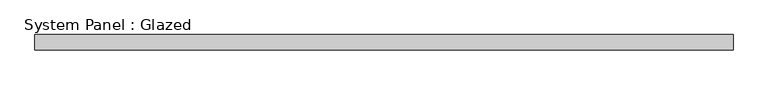
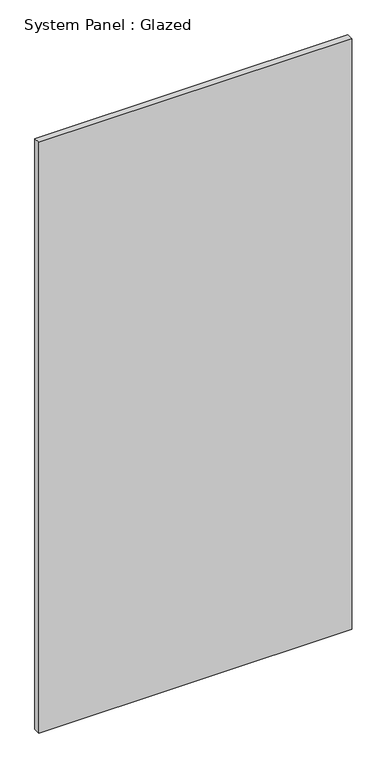
"""IFC4 building model written with IfcOpenShell, lengths in millimetres: plate geometry, System Panel : Glazed."""

from ifc_helpers import new_model, si_unit, origin, origin_with_axes, place, context, project, spatial, polyline, outline, extrude, source, transform, mapped, element, save


def system_panel_glazed_688a88ce(model_context):
    return source(origin(), model_context, "Body", "SweptSolid", [
        extrude(outline(polyline([(587.3750001, 19.05), (-587.3750001, 19.05), (-587.3750001, 44.45), (587.3750001, 44.45), (587.3750001, 19.05)])), origin_with_axes(), (0.0, 0.0, 1.0), 2343.15),
    ])


if __name__ == "__main__":
    model = new_model("IFC4")
    model_context = context("Model", 3, world=origin())
    ifc_project = project(units=[si_unit("LENGTHUNIT", "METRE", prefix="MILLI")], contexts=[model_context])
    site = spatial("IfcSite", under=ifc_project)
    building = spatial("IfcBuilding", under=site)
    placement = place(None, origin())
    system_panel_glazed_shape = system_panel_glazed_688a88ce(model_context)
    element("IfcPlate", 1, ObjectType="System Panel : Glazed", at=placement, inside=building, context=model_context, shape_type="MappedRepresentation", body=[
        mapped(system_panel_glazed_shape, transform((0.0, 0.0, 0.0), x_axis=(1.0, 0.0, 0.0), y_axis=(0.0, 1.0, 0.0), z_axis=(0.0, 0.0, 1.0))),
    ])
    save(model, "model.ifc")

# Revit data of these elements
# Type "System Panel : Glazed"
#   Construction Type Id = "GSP4R"
#   Analytic Construction = "1/8 in Pilkington single glazing"
#   Visual Light Transmittance = 0.9
#   Solar Heat Gain Coefficient = 0.86
#   Heat Transfer Coefficient (U) = 1.18115 BTU/(h·ft²·°F)
#   Define Thermal Properties by = 1
# Element 1 (IfcPlate, "System Panel : Glazed")
#   Materials on its faces: "Glass"
# Materials
#   "Glass": class "Glass", colour RGB 0 128 192, transparency 0.75, Description = "Soda Lime Glass", Cost = 0
